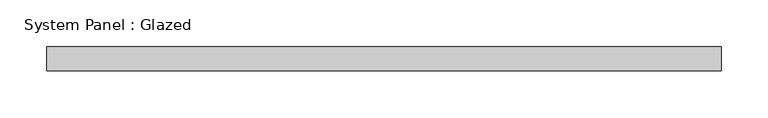
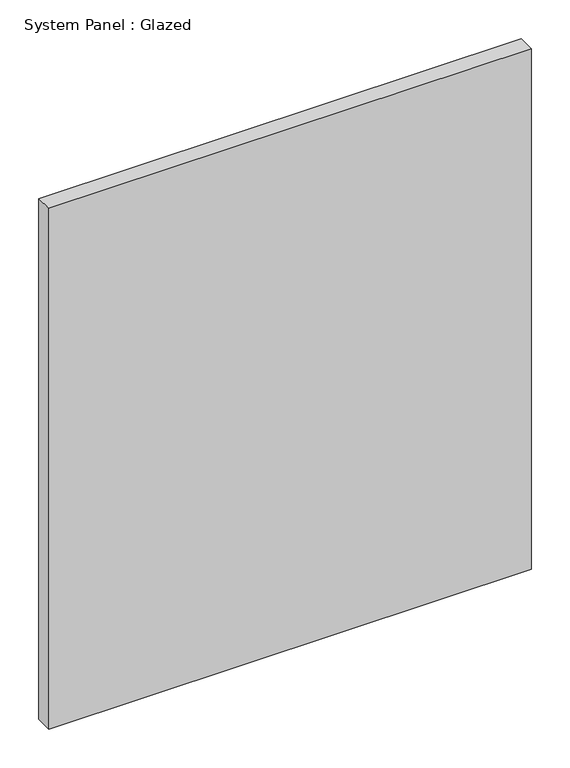
"""IFC4 building model written with IfcOpenShell, lengths in millimetres: plate geometry, System Panel : Glazed."""

from ifc_helpers import new_model, si_unit, origin, origin_with_axes, place, context, project, spatial, polyline, outline, extrude, source, transform, mapped, element, save


def system_panel_glazed_0825baf2(model_context):
    return source(origin(), model_context, "Body", "SweptSolid", [
        extrude(outline(polyline([(358.775, 19.05), (-358.775, 19.05), (-358.775, 44.45), (358.775, 44.45), (358.775, 19.05)])), origin_with_axes(), (0.0, 0.0, 1.0), 819.15),
    ])


if __name__ == "__main__":
    model = new_model("IFC4")
    model_context = context("Model", 3, world=origin())
    ifc_project = project(units=[si_unit("LENGTHUNIT", "METRE", prefix="MILLI")], contexts=[model_context])
    site = spatial("IfcSite", under=ifc_project)
    building = spatial("IfcBuilding", under=site)
    placement = place(None, origin())
    system_panel_glazed_shape = system_panel_glazed_0825baf2(model_context)
    element("IfcPlate", 1, ObjectType="System Panel : Glazed", at=placement, inside=building, context=model_context, shape_type="MappedRepresentation", body=[
        mapped(system_panel_glazed_shape, transform((0.0, 0.0, 0.0), x_axis=(1.0, 0.0, 0.0), y_axis=(0.0, 1.0, 0.0), z_axis=(0.0, 0.0, 1.0))),
    ])
    save(model, "model.ifc")

# Revit data of these elements
# Type "System Panel : Glazed"
#   Construction Type Id = "GSP4R"
#   Analytic Construction = "1/8 in Pilkington single glazing"
#   Visual Light Transmittance = 0.9
#   Solar Heat Gain Coefficient = 0.86
#   Heat Transfer Coefficient (U) = 1.18115 BTU/(h·ft²·°F)
#   Define Thermal Properties by = 1
# Element 1 (IfcPlate, "System Panel : Glazed")
#   Materials on its faces: "Glass"
# Materials
#   "Glass": class "Glass", colour RGB 0 128 192, transparency 0.75, Description = "Soda Lime Glass", Cost = 0
